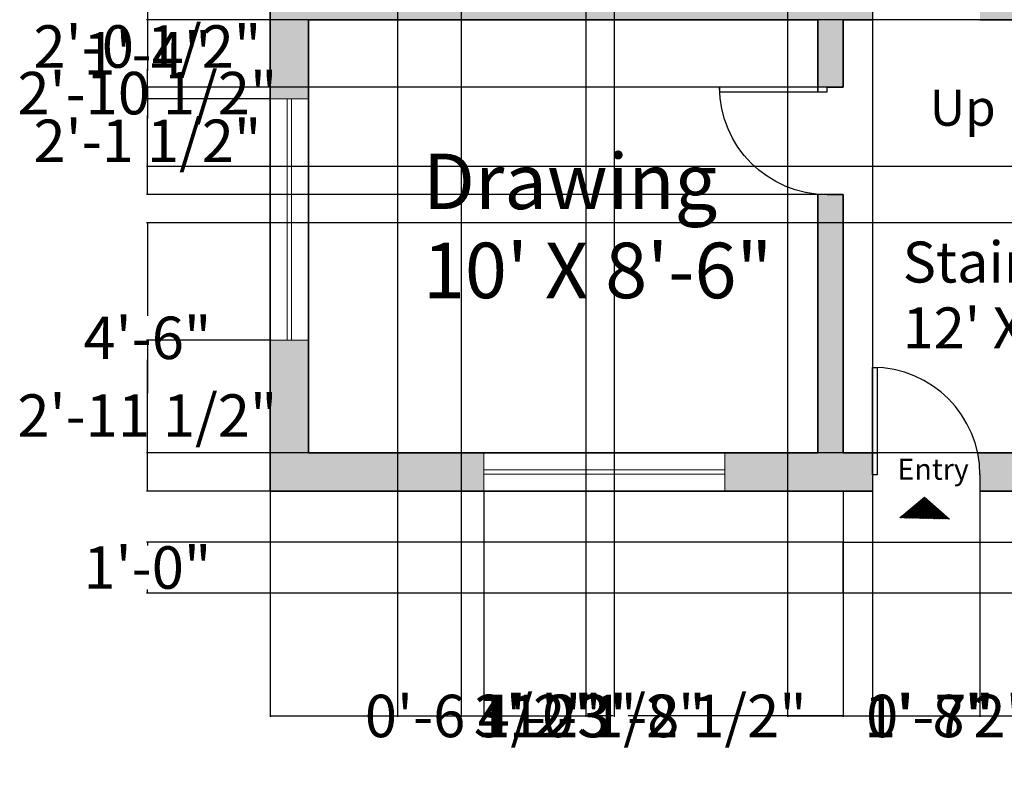
# Model space of a CAD drawing. Units: inches. Extents: x 46 to 946, y 121 to 740.
# Tile 1 of 4: x 55 to 287, y 121 to 299. Entities that reach past the tile are written whole.
import ezdxf

# ---------------------------------------------------------------- set-up
doc = ezdxf.new("R2010")
doc.units = ezdxf.units.IN
doc.header["$MEASUREMENT"] = 0
for name, color, linetype, lineweight in [('A-ANNO-DIMS', 2, 'Continuous', 18), ('A-ANNO-SYMB', 7, 'Continuous', 18), ('A-ANNO-TEXT', 7, 'Continuous', 18), ('A-AREA-IDEN', 7, 'Continuous', 25), ('A-DOOR', 3, 'Continuous', 25), ('A-FLOR-STRS', 7, 'Continuous', 25), ('A-GLAZ', 4, 'Continuous', 18), ('A-WALL', 7, 'Continuous', 35), ('A-WALL-PATT', 8, 'Continuous', 13)]:
    doc.layers.add(name, color=color, linetype=linetype, lineweight=lineweight)
doc.styles.get("Standard").update_dxf_attribs({"font": 'arial.ttf'})
doc.dimstyles.get("Standard").update_dxf_attribs({"dimtxt": 10, "dimasz": 0.18, "dimexe": 0.18, "dimexo": 0.0625, "dimgap": 0.09, "dimtad": 0, "dimtih": 1, "dimtoh": 1, "dimdec": 0, "dimzin": 0, "dimdsep": 46, "dimlunit": 3, "dimtxsty": 'Standard', "dimcen": 0.09, "dimadec": 0, "dimazin": 0, "dimtfac": 1, "dimtdec": 0, "dimtofl": 0, "dimtmove": 0, "dimatfit": 3, "dimfxl": 1, "dimtolj": 1, "dimtzin": 0, "dimarcsym": 0})

# ---------------------------------------------------------------- blocks, each defined once
blk = doc.blocks.new('*U3')
for p, q in [((0, 0), (0, -6)), ((40, 0), (40, -6))]:
    blk.add_line(p, q)
blk.add_lwpolyline([(0, 0), (0, 40), (1.75, 40), (1.75, 0)], close=True)
blk.add_arc((0, 0), 40, 0, 90)
blk = doc.blocks.new('WIN-56_82IN')
for p, q in [((9, 56.82), (0, 56.82)), ((0, 0), (0, 56.82)), ((4, 56.82), (4, 0)), ((5, 56.82), (5, 0)), ((9, 56.82), (9, 0)), ((9, 0), (0, 0))]:
    blk.add_line(p, q)
blk = doc.blocks.new('ARROW-DIRECTION')
h = blk.add_hatch()
h.set_pattern_fill('ANSI31', color=256, angle=180)
h.set_pattern_definition([(225, (391.19844, 225.63338), (0.088388348, -0.088388348), [])])
h.paths.add_polyline_path([(0, 0.27), (11.71, 0), (5.84, 5.18)])
for p, q in [((5.84, 5.18), (0, 0.27)), ((5.84, 5.18), (11.71, 0)), ((11.71, 0), (5.84, 5.18))]:
    blk.add_line(p, q)
blk = doc.blocks.new('*D24')
at = {"layer": 'A-ANNO-DIMS', "color": 0, "lineweight": -2, "transparency": 16777216}
for p, q in [((114.48, 188.4), (114.48, 135.33)), ((249.48, 164.4), (249.48, 135.33)), ((114.66, 135.51), (165.18, 135.51)), ((249.3, 135.51), (198.77, 135.51))]:
    blk.add_line(p, q, dxfattribs=at)
at = {"layer": 'A-ANNO-DIMS', "color": 0, "transparency": 16777216}
for points in [[(114.66, 135.54), (114.66, 135.48), (114.48, 135.51)], [(249.3, 135.54), (249.3, 135.48), (249.48, 135.51)]]:
    blk.add_solid(points, dxfattribs=at)
at = {"layer": 'Defpoints', "color": 0, "transparency": 16777216}
for p in [(114.48, 188.46), (249.48, 164.46), (249.48, 135.51)]:
    blk.add_point(p, dxfattribs=at)
at = {"layer": 'A-ANNO-DIMS', "color": 0, "transparency": 16777216, "insert": (181.98, 135.51), "char_height": 10, "attachment_point": 5}
blk.add_mtext('\\A1;11\'-3"', dxfattribs=at)
blk = doc.blocks.new('*D25')
at = {"layer": 'A-ANNO-DIMS', "color": 0, "lineweight": -2, "transparency": 16777216}
for p, q in [((249.48, 164.4), (249.48, 135.33)), ((296.21, 164.4), (296.21, 135.33)), ((249.66, 135.51), (296.03, 135.51)), ((296.21, 135.51), (296.39, 135.51))]:
    blk.add_line(p, q, dxfattribs=at)
at = {"layer": 'A-ANNO-DIMS', "color": 0, "transparency": 16777216}
for points in [[(249.66, 135.54), (249.66, 135.48), (249.48, 135.51)], [(296.03, 135.54), (296.03, 135.48), (296.21, 135.51)]]:
    blk.add_solid(points, dxfattribs=at)
at = {"layer": 'Defpoints', "color": 0, "transparency": 16777216}
for p in [(249.48, 164.46), (296.21, 164.46), (296.21, 135.51)]:
    blk.add_point(p, dxfattribs=at)
at = {"layer": 'A-ANNO-DIMS', "color": 0, "transparency": 16777216, "insert": (325.3, 135.51), "char_height": 10, "attachment_point": 5}
blk.add_mtext('\\A1;3\'-10 1/2"', dxfattribs=at)
blk = doc.blocks.new('*D31')
at = {"layer": 'A-ANNO-DIMS', "color": 0, "lineweight": -2, "transparency": 16777216}
for p, q in [((114.41, 224.01), (85.35, 224.01)), ((85.53, 223.83), (85.53, 211.5)), ((85.53, 188.64), (85.53, 200.97)), ((114.41, 188.46), (85.35, 188.46))]:
    blk.add_line(p, q, dxfattribs=at)
at = {"layer": 'A-ANNO-DIMS', "color": 0, "transparency": 16777216}
for points in [[(85.5, 223.83), (85.56, 223.83), (85.53, 224.01)], [(85.5, 188.64), (85.56, 188.64), (85.53, 188.46)]]:
    blk.add_solid(points, dxfattribs=at)
at = {"layer": 'Defpoints', "color": 0, "transparency": 16777216}
for p in [(85.53, 224.01), (114.48, 224.01), (114.48, 188.46)]:
    blk.add_point(p, dxfattribs=at)
at = {"layer": 'A-ANNO-DIMS', "color": 0, "transparency": 16777216, "insert": (85.53, 206.24), "char_height": 10, "attachment_point": 5}
blk.add_mtext('\\A1;2\'-11 1/2"', dxfattribs=at)
blk = doc.blocks.new('*D32')
at = {"layer": 'A-ANNO-DIMS', "color": 0, "lineweight": -2, "transparency": 16777216}
for p, q in [((123.41, 305.46), (85.35, 305.46)), ((85.53, 305.28), (85.53, 298.41)), ((85.53, 281.01), (85.53, 287.89)), ((114.41, 280.83), (85.35, 280.83))]:
    blk.add_line(p, q, dxfattribs=at)
at = {"layer": 'A-ANNO-DIMS', "color": 0, "transparency": 16777216}
for points in [[(85.5, 305.28), (85.56, 305.28), (85.53, 305.46)], [(85.5, 281.01), (85.56, 281.01), (85.53, 280.83)]]:
    blk.add_solid(points, dxfattribs=at)
at = {"layer": 'Defpoints', "color": 0, "transparency": 16777216}
for p in [(85.53, 305.46), (123.48, 305.46), (114.48, 280.83)]:
    blk.add_point(p, dxfattribs=at)
at = {"layer": 'A-ANNO-DIMS', "color": 0, "transparency": 16777216, "insert": (85.53, 293.15), "char_height": 10, "attachment_point": 5}
blk.add_mtext('\\A1;2\'-0 1/2"', dxfattribs=at)
blk = doc.blocks.new('*D43')
at = {"layer": 'A-ANNO-DIMS', "color": 0, "lineweight": -2, "transparency": 16777216}
for p, q in [((114.48, 188.4), (114.48, 135.33)), ((164.78, 188.4), (164.78, 135.33)), ((114.66, 135.51), (164.6, 135.51)), ((164.78, 135.51), (164.96, 135.51))]:
    blk.add_line(p, q, dxfattribs=at)
at = {"layer": 'A-ANNO-DIMS', "color": 0, "transparency": 16777216}
for points in [[(114.66, 135.54), (114.66, 135.48), (114.48, 135.51)], [(164.6, 135.54), (164.6, 135.48), (164.78, 135.51)]]:
    blk.add_solid(points, dxfattribs=at)
at = {"layer": 'Defpoints', "color": 0, "transparency": 16777216}
for p in [(114.48, 188.46), (164.78, 188.46), (164.78, 135.51)]:
    blk.add_point(p, dxfattribs=at)
at = {"layer": 'A-ANNO-DIMS', "color": 0, "transparency": 16777216, "insert": (190.2, 135.51), "char_height": 10, "attachment_point": 5}
blk.add_mtext('\\A1;4\'-2 1/2"', dxfattribs=at)
blk = doc.blocks.new('*D44')
at = {"layer": 'A-ANNO-DIMS', "color": 0, "lineweight": -2, "transparency": 16777216}
for p, q in [((256.37, 188.4), (256.37, 135.33)), ((281.69, 188.4), (281.69, 135.33)), ((256.55, 135.51), (281.51, 135.51)), ((281.69, 135.51), (281.87, 135.51))]:
    blk.add_line(p, q, dxfattribs=at)
at = {"layer": 'A-ANNO-DIMS', "color": 0, "transparency": 16777216}
for points in [[(256.55, 135.54), (256.55, 135.48), (256.37, 135.51)], [(281.51, 135.54), (281.51, 135.48), (281.69, 135.51)]]:
    blk.add_solid(points, dxfattribs=at)
at = {"layer": 'Defpoints', "color": 0, "transparency": 16777216}
for p in [(256.37, 188.46), (281.69, 188.46), (281.69, 135.51)]:
    blk.add_point(p, dxfattribs=at)
at = {"layer": 'A-ANNO-DIMS', "color": 0, "transparency": 16777216, "insert": (306.99, 135.51), "char_height": 10, "attachment_point": 5}
blk.add_mtext('\\A1;2\'-1 1/2"', dxfattribs=at)
blk = doc.blocks.new('*D47')
at = {"layer": 'A-ANNO-DIMS', "color": 0, "lineweight": -2, "transparency": 16777216}
for p, q in [((144.44, 436.91), (144.44, 135.33)), ((188.83, 436.91), (188.83, 135.33)), ((144.62, 135.51), (188.65, 135.51)), ((188.83, 135.51), (189.01, 135.51))]:
    blk.add_line(p, q, dxfattribs=at)
at = {"layer": 'A-ANNO-DIMS', "color": 0, "transparency": 16777216}
for points in [[(144.62, 135.54), (144.62, 135.48), (144.44, 135.51)], [(188.65, 135.54), (188.65, 135.48), (188.83, 135.51)]]:
    blk.add_solid(points, dxfattribs=at)
at = {"layer": 'Defpoints', "color": 0, "transparency": 16777216}
for p in [(144.44, 436.97), (188.83, 436.97), (188.83, 135.51)]:
    blk.add_point(p, dxfattribs=at)
at = {"layer": 'A-ANNO-DIMS', "color": 0, "transparency": 16777216, "insert": (214.03, 135.51), "char_height": 10, "attachment_point": 5}
blk.add_mtext('\\A1;3\'-8 1/2"', dxfattribs=at)
blk = doc.blocks.new('*D49')
at = {"layer": 'A-ANNO-DIMS', "color": 0, "lineweight": -2, "transparency": 16777216}
for p, q in [((159.48, 460.26), (159.48, 135.33)), ((195.48, 460.26), (195.48, 135.33)), ((159.66, 135.51), (164.1, 135.51)), ((195.3, 135.51), (190.85, 135.51))]:
    blk.add_line(p, q, dxfattribs=at)
at = {"layer": 'A-ANNO-DIMS', "color": 0, "transparency": 16777216}
for points in [[(159.66, 135.54), (159.66, 135.48), (159.48, 135.51)], [(195.3, 135.54), (195.3, 135.48), (195.48, 135.51)]]:
    blk.add_solid(points, dxfattribs=at)
at = {"layer": 'Defpoints', "color": 0, "transparency": 16777216}
for p in [(159.48, 460.32), (195.48, 460.32), (195.48, 135.51)]:
    blk.add_point(p, dxfattribs=at)
at = {"layer": 'A-ANNO-DIMS', "color": 0, "transparency": 16777216, "insert": (177.48, 135.51), "char_height": 10, "attachment_point": 5}
blk.add_mtext('\\A1;3\'-0"', dxfattribs=at)
blk = doc.blocks.new('*D51')
at = {"layer": 'A-ANNO-DIMS', "color": 0, "lineweight": -2, "transparency": 16777216}
for p, q in [((249.48, 188.4), (249.48, 135.33)), ((256.37, 188.4), (256.37, 135.33)), ((249.66, 135.51), (256.19, 135.51)), ((256.37, 135.51), (256.55, 135.51))]:
    blk.add_line(p, q, dxfattribs=at)
at = {"layer": 'A-ANNO-DIMS', "color": 0, "transparency": 16777216}
for points in [[(249.66, 135.54), (249.66, 135.48), (249.48, 135.51)], [(256.19, 135.54), (256.19, 135.48), (256.37, 135.51)]]:
    blk.add_solid(points, dxfattribs=at)
at = {"layer": 'Defpoints', "color": 0, "transparency": 16777216}
for p in [(249.48, 188.46), (256.37, 188.46), (256.37, 135.51)]:
    blk.add_point(p, dxfattribs=at)
at = {"layer": 'A-ANNO-DIMS', "color": 0, "transparency": 16777216, "insert": (269.93, 135.51), "char_height": 10, "attachment_point": 5}
blk.add_mtext('\\A1;0\'-7"', dxfattribs=at)
blk = doc.blocks.new('*D52')
at = {"layer": 'A-ANNO-DIMS', "color": 0, "lineweight": -2, "transparency": 16777216}
for p, q in [((249.41, 176.46), (85.35, 176.46)), ((85.53, 176.28), (85.53, 175.66)), ((85.53, 164.64), (85.53, 165.27)), ((249.41, 164.46), (85.35, 164.46))]:
    blk.add_line(p, q, dxfattribs=at)
at = {"layer": 'A-ANNO-DIMS', "color": 0, "transparency": 16777216}
for points in [[(85.5, 176.28), (85.56, 176.28), (85.53, 176.46)], [(85.5, 164.64), (85.56, 164.64), (85.53, 164.46)]]:
    blk.add_solid(points, dxfattribs=at)
at = {"layer": 'Defpoints', "color": 0, "transparency": 16777216}
for p in [(249.48, 176.46), (85.53, 164.46), (249.48, 164.46)]:
    blk.add_point(p, dxfattribs=at)
at = {"layer": 'A-ANNO-DIMS', "color": 0, "transparency": 16777216, "insert": (85.53, 170.46), "char_height": 10, "attachment_point": 5}
blk.add_mtext('\\A1;1\'-0"', dxfattribs=at)
blk = doc.blocks.new('*D53')
at = {"layer": 'A-ANNO-DIMS', "color": 0, "lineweight": -2, "transparency": 16777216}
for p, q in [((249.41, 299.46), (85.35, 299.46)), ((85.53, 299.28), (85.53, 296.64)), ((85.53, 283.78), (85.53, 286.42)), ((249.41, 283.6), (85.35, 283.6))]:
    blk.add_line(p, q, dxfattribs=at)
at = {"layer": 'A-ANNO-DIMS', "color": 0, "transparency": 16777216}
for points in [[(85.5, 299.28), (85.56, 299.28), (85.53, 299.46)], [(85.5, 283.78), (85.56, 283.78), (85.53, 283.6)]]:
    blk.add_solid(points, dxfattribs=at)
at = {"layer": 'Defpoints', "color": 0, "transparency": 16777216}
for p in [(249.48, 299.46), (85.53, 283.6), (249.48, 283.6)]:
    blk.add_point(p, dxfattribs=at)
at = {"layer": 'A-ANNO-DIMS', "color": 0, "transparency": 16777216, "insert": (85.53, 291.53), "char_height": 10, "attachment_point": 5}
blk.add_mtext('\\A1;1\'-4"', dxfattribs=at)
blk = doc.blocks.new('*D54')
at = {"layer": 'A-ANNO-DIMS', "color": 0, "lineweight": -2, "transparency": 16777216}
for p, q in [((249.41, 283.6), (85.35, 283.6)), ((85.53, 283.42), (85.53, 276.2)), ((85.53, 258.46), (85.53, 265.68)), ((249.41, 258.28), (85.35, 258.28))]:
    blk.add_line(p, q, dxfattribs=at)
at = {"layer": 'A-ANNO-DIMS', "color": 0, "transparency": 16777216}
for points in [[(85.5, 283.42), (85.56, 283.42), (85.53, 283.6)], [(85.5, 258.46), (85.56, 258.46), (85.53, 258.28)]]:
    blk.add_solid(points, dxfattribs=at)
at = {"layer": 'Defpoints', "color": 0, "transparency": 16777216}
for p in [(249.48, 283.6), (85.53, 258.28), (249.48, 258.28)]:
    blk.add_point(p, dxfattribs=at)
at = {"layer": 'A-ANNO-DIMS', "color": 0, "transparency": 16777216, "insert": (85.53, 270.94), "char_height": 10, "attachment_point": 5}
blk.add_mtext('\\A1;2\'-1 1/2"', dxfattribs=at)
blk = doc.blocks.new('*D55')
at = {"layer": 'A-ANNO-DIMS', "color": 0, "lineweight": -2, "transparency": 16777216}
for p, q in [((307.8, 299.46), (85.35, 299.46)), ((85.53, 299.28), (85.53, 287.43)), ((85.53, 265.06), (85.53, 276.91)), ((307.8, 264.88), (85.35, 264.88))]:
    blk.add_line(p, q, dxfattribs=at)
at = {"layer": 'A-ANNO-DIMS', "color": 0, "transparency": 16777216}
for points in [[(85.5, 299.28), (85.56, 299.28), (85.53, 299.46)], [(85.5, 265.06), (85.56, 265.06), (85.53, 264.88)]]:
    blk.add_solid(points, dxfattribs=at)
at = {"layer": 'Defpoints', "color": 0, "transparency": 16777216}
for p in [(307.86, 299.46), (85.53, 264.88), (307.86, 264.88)]:
    blk.add_point(p, dxfattribs=at)
at = {"layer": 'A-ANNO-DIMS', "color": 0, "transparency": 16777216, "insert": (85.53, 282.17), "char_height": 10, "attachment_point": 5}
blk.add_mtext('\\A1;2\'-10 1/2"', dxfattribs=at)
blk = doc.blocks.new('*D57')
at = {"layer": 'A-ANNO-DIMS', "color": 0, "lineweight": -2, "transparency": 16777216}
for p, q in [((327.41, 251.63), (85.35, 251.63)), ((85.53, 251.45), (85.53, 229.74)), ((85.53, 197.64), (85.53, 219.35)), ((327.41, 197.46), (85.35, 197.46))]:
    blk.add_line(p, q, dxfattribs=at)
at = {"layer": 'A-ANNO-DIMS', "color": 0, "transparency": 16777216}
for points in [[(85.5, 251.45), (85.56, 251.45), (85.53, 251.63)], [(85.5, 197.64), (85.56, 197.64), (85.53, 197.46)]]:
    blk.add_solid(points, dxfattribs=at)
at = {"layer": 'Defpoints', "color": 0, "transparency": 16777216}
for p in [(327.48, 251.63), (85.53, 197.46), (327.48, 197.46)]:
    blk.add_point(p, dxfattribs=at)
at = {"layer": 'A-ANNO-DIMS', "color": 0, "transparency": 16777216, "insert": (85.53, 224.55), "char_height": 10, "attachment_point": 5}
blk.add_mtext('\\A1;4\'-6"', dxfattribs=at)
blk = doc.blocks.new('*D64')
at = {"layer": 'A-ANNO-DIMS', "color": 0, "lineweight": -2, "transparency": 16777216}
for p, q in [((188.83, 436.91), (188.83, 135.33)), ((195.48, 432.4), (195.48, 135.33)), ((188.83, 135.51), (188.65, 135.51)), ((195.3, 135.51), (189.01, 135.51))]:
    blk.add_line(p, q, dxfattribs=at)
at = {"layer": 'A-ANNO-DIMS', "color": 0, "transparency": 16777216}
for points in [[(189.01, 135.54), (189.01, 135.48), (188.83, 135.51)], [(195.3, 135.54), (195.3, 135.48), (195.48, 135.51)]]:
    blk.add_solid(points, dxfattribs=at)
at = {"layer": 'Defpoints', "color": 0, "transparency": 16777216}
for p in [(188.83, 436.97), (195.48, 432.46), (188.83, 135.51)]:
    blk.add_point(p, dxfattribs=at)
at = {"layer": 'A-ANNO-DIMS', "color": 0, "transparency": 16777216, "insert": (163.61, 135.51), "char_height": 10, "attachment_point": 5}
blk.add_mtext('\\A1;0\'-6 1/2"', dxfattribs=at)
blk = doc.blocks.new('*D70')
at = {"layer": 'A-ANNO-DIMS', "color": 0, "lineweight": -2, "transparency": 16777216}
for p, q in [((236.36, 528.4), (236.36, 135.33)), ((256.37, 528.4), (256.37, 135.33)), ((236.54, 135.51), (256.19, 135.51)), ((256.37, 135.51), (256.55, 135.51))]:
    blk.add_line(p, q, dxfattribs=at)
at = {"layer": 'A-ANNO-DIMS', "color": 0, "transparency": 16777216}
for points in [[(236.54, 135.54), (236.54, 135.48), (236.36, 135.51)], [(256.19, 135.54), (256.19, 135.48), (256.37, 135.51)]]:
    blk.add_solid(points, dxfattribs=at)
at = {"layer": 'Defpoints', "color": 0, "transparency": 16777216}
for p in [(236.36, 528.46), (256.37, 528.46), (256.37, 135.51)]:
    blk.add_point(p, dxfattribs=at)
at = {"layer": 'A-ANNO-DIMS', "color": 0, "transparency": 16777216, "insert": (269.46, 135.51), "char_height": 10, "attachment_point": 5}
blk.add_mtext('\\A1;1\'-8"', dxfattribs=at)

msp = doc.modelspace()

# ---------------------------------------------------------------- hatches: boundary and pattern name
at = {"layer": 'A-WALL-PATT'}
h = msp.add_hatch(color=256, dxfattribs=at)
h.dxf.hatch_style = 1
h.paths.add_polyline_path([(256.37, 197.46), (249.48, 197.46), (249.48, 258.28), (245.68, 258.28, -0.021769), (243.48, 258.37), (243.48, 197.46), (221.61, 197.46), (221.61, 188.46), (243.48, 188.46), (256.37, 188.46), (256.37, 192.26)])
h.paths.add_polyline_path([(164.78, 197.46), (123.48, 197.46), (123.48, 224.01), (114.48, 224.01), (114.48, 188.46), (164.78, 188.46)])
h.paths.add_polyline_path([(402.48, 216.63), (393.48, 216.63), (393.48, 197.46), (327.48, 197.46), (281.15, 197.46, -0.051771), (281.69, 192.26), (281.69, 188.46), (402.48, 188.46)])
h.paths.add_polyline_path([(123.48, 346.49), (114.48, 346.49), (114.48, 280.83), (123.48, 280.83), (123.48, 299.46), (243.48, 299.46), (243.48, 283.6), (245.68, 283.6), (249.48, 283.6), (249.48, 299.46), (256.37, 299.46), (256.37, 303.26), (256.37, 304.46), (249.48, 304.46), (249.48, 432.46), (243.48, 432.46), (232.61, 432.46), (232.61, 426.46), (243.48, 426.46), (243.48, 305.46), (123.48, 305.46)])
h.paths.add_polyline_path([(231.5, 428.66), (232.61, 428.66), (232.61, 403.34), (231.5, 403.34), (231.5, 403.37, -0.376395), (207.38, 426.46), (123.48, 426.46), (123.48, 403.31), (114.48, 403.31), (114.48, 453.42), (123.48, 453.42), (123.48, 432.46), (195.48, 432.46), (195.48, 474.9), (201.48, 474.9), (201.48, 432.46), (207.29, 432.46), (207.29, 428.66, 0.401453), (231.5, 403.37)])
h.paths.add_polyline_path([(211.14, 534.46), (123.48, 534.46), (123.48, 573.18), (114.48, 573.18), (114.48, 510.24), (123.48, 510.24), (123.48, 528.46), (195.48, 528.46), (195.48, 495.84), (201.48, 495.84), (201.48, 528.46), (211.04, 528.46), (211.04, 532.26, -0.021769)])
h.paths.add_polyline_path([(123.48, 684.46), (243.48, 684.46), (243.48, 534.46), (236.36, 534.46), (236.36, 532.26), (236.36, 528.46), (256.37, 528.46), (256.37, 532.26), (256.37, 534.46), (249.48, 534.46), (249.48, 684.46), (393.48, 684.46), (393.48, 647.42), (402.48, 647.42), (402.48, 693.46), (114.48, 693.46), (114.48, 630), (123.48, 630)])
h.paths.add_polyline_path([(402.48, 590.59), (393.48, 590.59), (393.48, 534.46), (281.59, 534.46, -0.021769), (281.69, 532.26), (281.69, 528.46), (298.48, 528.46), (298.48, 518.41), (302.28, 518.41), (304.48, 518.41), (304.48, 528.46), (393.48, 528.46), (393.48, 518.87), (402.48, 518.87)])
h.paths.add_polyline_path([(402.48, 500.87), (393.48, 500.87), (393.48, 482.46), (304.48, 482.46), (304.48, 493.19, -0.021769), (302.28, 493.09), (298.48, 493.09), (298.48, 482.46), (298.48, 476.46), (304.48, 476.46), (393.48, 476.46), (393.48, 455.17), (402.48, 455.17)])
h.paths.add_polyline_path([(402.48, 419.17), (393.48, 419.17), (393.48, 356.8), (402.48, 356.8)])
h.paths.add_polyline_path([(358.48, 304.46), (281.66, 304.46, -0.01187), (281.69, 303.26), (281.69, 299.46), (358.48, 299.46)])

# ---------------------------------------------------------------- linework, layer by layer
at = {"layer": 'A-FLOR-STRS'}
for p, q in [((249.48, 188.46), (249.48, 176.46)), ((249.48, 176.46), (296.21, 176.46)), ((249.48, 164.46), (249.48, 176.46)), ((296.21, 164.46), (249.48, 164.46))]:
    msp.add_line(p, q, dxfattribs=at)
at = {"layer": 'A-WALL'}
for p, q in [((114.48, 693.46), (114.48, 188.46)), ((123.48, 299.46), (123.48, 197.46)), ((123.48, 299.46), (243.48, 299.46)), ((243.48, 299.46), (243.48, 282.49)), ((243.48, 299.46), (243.48, 282.49)), ((249.48, 299.46), (249.48, 283.6)), ((249.48, 299.46), (256.37, 299.46)), ((281.69, 299.46), (393.48, 299.46)), ((243.48, 258.37), (243.48, 197.46)), ((243.48, 258.37), (243.48, 197.46)), ((249.48, 258.28), (249.48, 197.46)), ((243.48, 197.46), (123.48, 197.46)), ((123.48, 197.46), (243.48, 197.46)), ((249.48, 197.46), (257.48, 197.46)), ((281.15, 197.46), (393.48, 197.46)), ((114.48, 188.46), (243.48, 188.46)), ((243.48, 188.46), (256.37, 188.46)), ((249.48, 188.46), (256.37, 188.46)), ((281.69, 188.46), (402.48, 188.46)), ((281.69, 188.46), (393.48, 188.46))]:
    msp.add_line(p, q, dxfattribs=at)

# ---------------------------------------------------------------- block references
at = {"layer": 'A-ANNO-SYMB'}
msp.add_blockref('ARROW-DIRECTION', (262.79, 181.88), dxfattribs=at)
at = {"layer": 'A-DOOR', "xscale": -0.6330408260540115, "yscale": 0.6330408260540115, "zscale": 0.6330408260540115, "rotation": 90.00000000000007}
msp.add_blockref('*U3', (245.68, 283.6), dxfattribs=at)
at = {"layer": 'A-DOOR', "xscale": 0.6330408260540115, "yscale": 0.6330408260540115, "zscale": 0.6330408260540115}
msp.add_blockref('*U3', (256.37, 192.26), dxfattribs=at)
at = {"layer": 'A-GLAZ'}
msp.add_blockref('WIN-56_82IN', (114.48, 224.01), dxfattribs=at)
at = {"layer": 'A-GLAZ', "rotation": 270}
msp.add_blockref('WIN-56_82IN', (164.78, 197.46), dxfattribs=at)

# ---------------------------------------------------------------- texts
at = {"layer": 'A-ANNO-TEXT'}
for s, height, p in [('Up', 8.494, (269.86, 274.5)), ('Entry', 4.954, (262.26, 191.13))]:
    msp.add_text(s, height=height, dxfattribs=at).set_placement(p)
at = {"layer": 'A-AREA-IDEN'}
for s, height, p in [('Drawing', 13.067, (150.45, 254.87)), ('10\' X 8\'-6"', 13.0671, (150.45, 233.88)), ('Stair case', 9.654, (263.48, 237.57)), ('12\' X 8\'-6"', 9.6537, (263.48, 222.06))]:
    msp.add_text(s, height=height, dxfattribs=at).set_placement(p)

# ---------------------------------------------------------------- dimensions: what is measured, and where the dimension line sits
at = {"layer": 'A-ANNO-DIMS'}
for base, p1, p2, picture, middle in [((256.37, 135.51), (236.36, 528.46), (256.37, 528.46), '*D70', (269.46, 135.51)), ((195.48, 135.51), (159.48, 460.32), (195.48, 460.32), '*D49', (177.48, 135.51)), ((188.8251, 135.5113), (195.4768, 432.4613), (188.8251, 436.9697), '*D64', (163.6131, 135.5113)), ((188.83, 135.51), (144.44, 436.97), (188.83, 436.97), '*D47', (214.03, 135.51)), ((249.48, 135.51), (114.48, 188.46), (249.48, 164.46), '*D24', (181.98, 135.51)), ((164.78, 135.51), (114.48, 188.46), (164.78, 188.46), '*D43', (190.2, 135.51)), ((256.37, 135.51), (249.48, 188.46), (256.37, 188.46), '*D51', (269.93, 135.51)), ((281.69, 135.51), (256.37, 188.46), (281.69, 188.46), '*D44', (306.99, 135.51)), ((296.21, 135.51), (249.48, 164.46), (296.21, 164.46), '*D25', (325.3, 135.51))]:
    dim = msp.add_linear_dim(base=base, p1=p1, p2=p2, dimstyle='Standard', override={"dimdec": 1, "dimlfac": 1, "dimrnd": 0, "dimzin": 1, "dimdsep": 46, "dimlunit": 4, "dimfrac": 2}, dxfattribs=at)
    dim.commit()
    dim.dimension.update_dxf_attribs({"geometry": picture, "text_midpoint": middle})
for base, p1, p2, picture, middle in [((85.53, 305.46), (114.48, 280.83), (123.48, 305.46), '*D32', (85.53, 293.15)), ((85.53, 264.88), (307.86, 299.46), (307.86, 264.88), '*D55', (85.53, 282.17)), ((85.53, 283.6), (249.48, 299.46), (249.48, 283.6), '*D53', (85.53, 291.53)), ((85.53, 258.28), (249.48, 283.6), (249.48, 258.28), '*D54', (85.53, 270.94)), ((85.53, 197.46), (327.48, 251.63), (327.48, 197.46), '*D57', (85.53, 224.55)), ((85.5268, 224.0089), (114.4768, 188.4613), (114.4768, 224.0089), '*D31', (85.5268, 206.2351)), ((85.53, 164.46), (249.48, 176.46), (249.48, 164.46), '*D52', (85.53, 170.46))]:
    dim = msp.add_linear_dim(base=base, p1=p1, p2=p2, angle=90, dimstyle='Standard', override={"dimdec": 1, "dimlfac": 1, "dimrnd": 0, "dimzin": 1, "dimdsep": 46, "dimlunit": 4, "dimfrac": 2}, dxfattribs=at)
    dim.commit()
    dim.dimension.update_dxf_attribs({"geometry": picture, "text_midpoint": middle})

doc.saveas('drawing.dxf')
